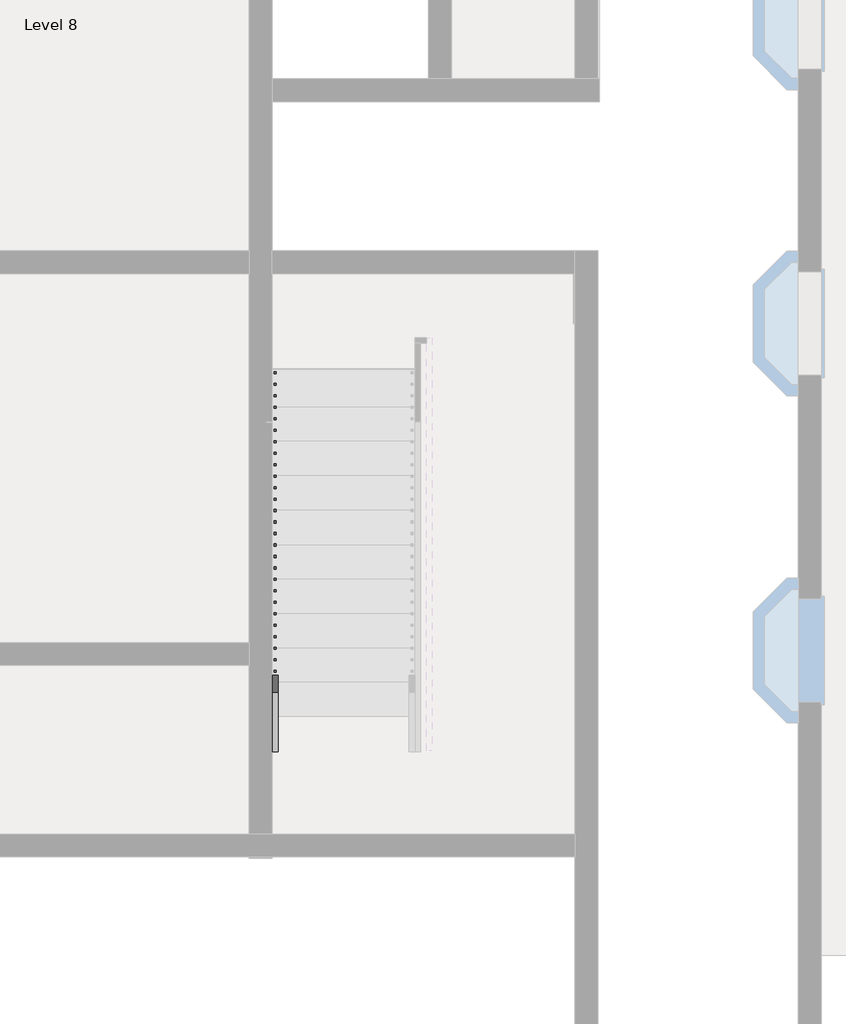
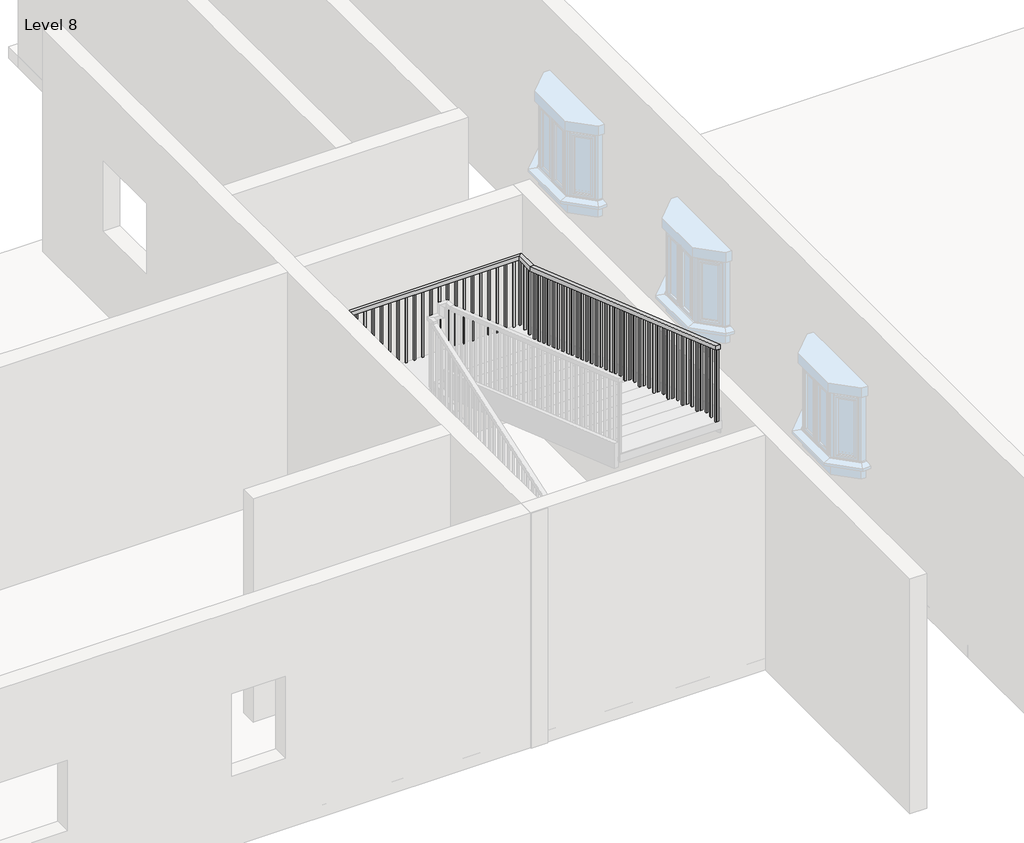
# One storey, part 8 of 14: 1 railing.
"""IFC4 building model written with IfcOpenShell, lengths in millimetres."""

from ifc_helpers import new_model, si_unit, frame, origin, place, context, project, spatial, polyline, outline, extrude, faceted_brep, element, save

model = new_model("IFC4")

# Units and contexts
model_context = context("Model", 3, world=origin())
ifc_project = project(units=[si_unit("LENGTHUNIT", "METRE", prefix="MILLI")], contexts=[model_context])

# Site, building, storey
site = spatial("IfcSite", under=ifc_project)
building = spatial("IfcBuilding", under=site)
storey = spatial("IfcBuildingStorey", under=building, Name="Level 8", Elevation=21336.0)

# Railing
placement = place(None, origin())
element("IfcRailing", 1, ObjectType="Handrail - Rectangular", at=placement, inside=storey, context=model_context, shape_type="SolidModel", body=[
    faceted_brep([(-3857.687215, -9955.5916506, 22355.9076923), (-3857.687215, -9955.5916506, 22302.1602476), (-3806.887215, -9955.5916506, 22302.1602476), (-3806.887215, -9955.5916506, 22355.9076923), (-3857.687215, -6291.6416506, 23622.0), (-3857.687215, -6283.1120276, 23571.2), (-3806.887215, -6283.1120276, 23571.2), (-3806.887215, -6291.6416506, 23622.0), (-3857.687215, -5713.7916506, 23622.0), (-3857.687215, -5713.7916506, 23571.2), (-3806.887215, -5764.5916506, 23571.2), (-3806.887215, -5764.5916506, 23622.0), (-1190.687215, -5713.7916506, 23622.0), (-1190.687215, -5713.7916506, 23571.2), (-1241.487215, -5764.5916506, 23571.2), (-1241.487215, -5764.5916506, 23622.0), (-1190.687215, -5986.8416506, 23622.0), (-1190.687215, -5995.3852679, 23571.2), (-1241.487215, -5995.3852679, 23571.2), (-1241.487215, -5986.8416506, 23622.0), (-1190.687215, -9949.2416506, 24993.6), (-1241.487215, -9949.2416506, 24993.6), (-1241.487215, -9949.2416506, 24939.842594), (-1190.687215, -9949.2416506, 24939.842594)], [[[0, 1, 2, 3]], [[1, 0, 4, 5]], [[2, 1, 5, 6]], [[3, 2, 6, 7]], [[0, 3, 7, 4]], [[5, 4, 8, 9]], [[6, 5, 9, 10]], [[7, 6, 10, 11]], [[4, 7, 11, 8]], [[9, 8, 12, 13]], [[10, 9, 13, 14]], [[11, 10, 14, 15]], [[8, 11, 15, 12]], [[13, 12, 16, 17]], [[14, 13, 17, 18]], [[15, 14, 18, 19]], [[12, 15, 19, 16]], [[20, 21, 22, 23]], [[17, 16, 20, 23]], [[18, 17, 23, 22]], [[19, 18, 22, 21]], [[16, 19, 21, 20]]]),
    extrude(outline(polyline([(-9895.2666506, 24921.1589402), (-9895.2666506, 23973.6923077), (-9914.3166506, 23973.6923077), (-9914.3166506, 24927.7531709), (-9895.2666506, 24921.1589402)])), frame((-1225.612215, 0.0, 0.0), z_axis=(1.0, 0.0, 0.0), x_axis=(0.0, 1.0, 0.0)), (0.0, 0.0, 1.0), 19.05),
    extrude(outline(polyline([(-9793.6666506, 24885.9897094), (-9793.6666506, 23973.6923077), (-9812.7166506, 23973.6923077), (-9812.7166506, 24892.5839402), (-9793.6666506, 24885.9897094)])), frame((-1225.612215, 0.0, 0.0), z_axis=(1.0, 0.0, 0.0), x_axis=(0.0, 1.0, 0.0)), (0.0, 0.0, 1.0), 19.05),
    extrude(outline(polyline([(-9692.0666506, 24850.8204786), (-9692.0666506, 23973.6923077), (-9711.1166506, 23973.6923077), (-9711.1166506, 24857.4147094), (-9692.0666506, 24850.8204786)])), frame((-1225.612215, 0.0, 0.0), z_axis=(1.0, 0.0, 0.0), x_axis=(0.0, 1.0, 0.0)), (0.0, 0.0, 1.0), 19.05),
    extrude(outline(polyline([(-9590.4666506, 24815.6512479), (-9590.4666506, 23868.1846154), (-9609.5166506, 23868.1846154), (-9609.5166506, 24822.2454786), (-9590.4666506, 24815.6512479)])), frame((-1225.612215, 0.0, 0.0), z_axis=(1.0, 0.0, 0.0), x_axis=(0.0, 1.0, 0.0)), (0.0, 0.0, 1.0), 19.05),
    extrude(outline(polyline([(-9488.8666506, 24780.4820171), (-9488.8666506, 23868.1846154), (-9507.9166506, 23868.1846154), (-9507.9166506, 24787.0762479), (-9488.8666506, 24780.4820171)])), frame((-1225.612215, 0.0, 0.0), z_axis=(1.0, 0.0, 0.0), x_axis=(0.0, 1.0, 0.0)), (0.0, 0.0, 1.0), 19.05),
    extrude(outline(polyline([(-9387.2666506, 24745.3127863), (-9387.2666506, 23868.1846154), (-9406.3166506, 23868.1846154), (-9406.3166506, 24751.9070171), (-9387.2666506, 24745.3127863)])), frame((-1225.612215, 0.0, 0.0), z_axis=(1.0, 0.0, 0.0), x_axis=(0.0, 1.0, 0.0)), (0.0, 0.0, 1.0), 19.05),
    extrude(outline(polyline([(-9285.6666506, 24710.1435556), (-9285.6666506, 23762.6769231), (-9304.7166506, 23762.6769231), (-9304.7166506, 24716.7377863), (-9285.6666506, 24710.1435556)])), frame((-1225.612215, 0.0, 0.0), z_axis=(1.0, 0.0, 0.0), x_axis=(0.0, 1.0, 0.0)), (0.0, 0.0, 1.0), 19.05),
    extrude(outline(polyline([(-9184.0666506, 24674.9743248), (-9184.0666506, 23762.6769231), (-9203.1166506, 23762.6769231), (-9203.1166506, 24681.5685556), (-9184.0666506, 24674.9743248)])), frame((-1225.612215, 0.0, 0.0), z_axis=(1.0, 0.0, 0.0), x_axis=(0.0, 1.0, 0.0)), (0.0, 0.0, 1.0), 19.05),
    extrude(outline(polyline([(-9082.4666506, 24639.805094), (-9082.4666506, 23762.6769231), (-9101.5166506, 23762.6769231), (-9101.5166506, 24646.3993248), (-9082.4666506, 24639.805094)])), frame((-1225.612215, 0.0, 0.0), z_axis=(1.0, 0.0, 0.0), x_axis=(0.0, 1.0, 0.0)), (0.0, 0.0, 1.0), 19.05),
    extrude(outline(polyline([(-8980.8666506, 24604.6358632), (-8980.8666506, 23657.1692308), (-8999.9166506, 23657.1692308), (-8999.9166506, 24611.230094), (-8980.8666506, 24604.6358632)])), frame((-1225.612215, 0.0, 0.0), z_axis=(1.0, 0.0, 0.0), x_axis=(0.0, 1.0, 0.0)), (0.0, 0.0, 1.0), 19.05),
    extrude(outline(polyline([(-8879.2666506, 24569.4666325), (-8879.2666506, 23657.1692308), (-8898.3166506, 23657.1692308), (-8898.3166506, 24576.0608632), (-8879.2666506, 24569.4666325)])), frame((-1225.612215, 0.0, 0.0), z_axis=(1.0, 0.0, 0.0), x_axis=(0.0, 1.0, 0.0)), (0.0, 0.0, 1.0), 19.05),
    extrude(outline(polyline([(-8777.6666506, 24534.2974017), (-8777.6666506, 23657.1692308), (-8796.7166506, 23657.1692308), (-8796.7166506, 24540.8916325), (-8777.6666506, 24534.2974017)])), frame((-1225.612215, 0.0, 0.0), z_axis=(1.0, 0.0, 0.0), x_axis=(0.0, 1.0, 0.0)), (0.0, 0.0, 1.0), 19.05),
    extrude(outline(polyline([(-8676.0666506, 24499.1281709), (-8676.0666506, 23551.6615385), (-8695.1166506, 23551.6615385), (-8695.1166506, 24505.7224017), (-8676.0666506, 24499.1281709)])), frame((-1225.612215, 0.0, 0.0), z_axis=(1.0, 0.0, 0.0), x_axis=(0.0, 1.0, 0.0)), (0.0, 0.0, 1.0), 19.05),
    extrude(outline(polyline([(-8574.4666506, 24463.9589402), (-8574.4666506, 23551.6615385), (-8593.5166506, 23551.6615385), (-8593.5166506, 24470.5531709), (-8574.4666506, 24463.9589402)])), frame((-1225.612215, 0.0, 0.0), z_axis=(1.0, 0.0, 0.0), x_axis=(0.0, 1.0, 0.0)), (0.0, 0.0, 1.0), 19.05),
    extrude(outline(polyline([(-8472.8666506, 24428.7897094), (-8472.8666506, 23551.6615385), (-8491.9166506, 23551.6615385), (-8491.9166506, 24435.3839402), (-8472.8666506, 24428.7897094)])), frame((-1225.612215, 0.0, 0.0), z_axis=(1.0, 0.0, 0.0), x_axis=(0.0, 1.0, 0.0)), (0.0, 0.0, 1.0), 19.05),
    extrude(outline(polyline([(-8371.2666506, 24393.6204786), (-8371.2666506, 23446.1538462), (-8390.3166506, 23446.1538462), (-8390.3166506, 24400.2147094), (-8371.2666506, 24393.6204786)])), frame((-1225.612215, 0.0, 0.0), z_axis=(1.0, 0.0, 0.0), x_axis=(0.0, 1.0, 0.0)), (0.0, 0.0, 1.0), 19.05),
    extrude(outline(polyline([(-8269.6666506, 24358.4512479), (-8269.6666506, 23446.1538462), (-8288.7166506, 23446.1538462), (-8288.7166506, 24365.0454786), (-8269.6666506, 24358.4512479)])), frame((-1225.612215, 0.0, 0.0), z_axis=(1.0, 0.0, 0.0), x_axis=(0.0, 1.0, 0.0)), (0.0, 0.0, 1.0), 19.05),
    extrude(outline(polyline([(-8168.0666506, 24323.2820171), (-8168.0666506, 23446.1538462), (-8187.1166506, 23446.1538462), (-8187.1166506, 24329.8762479), (-8168.0666506, 24323.2820171)])), frame((-1225.612215, 0.0, 0.0), z_axis=(1.0, 0.0, 0.0), x_axis=(0.0, 1.0, 0.0)), (0.0, 0.0, 1.0), 19.05),
    extrude(outline(polyline([(-8066.4666506, 24288.1127863), (-8066.4666506, 23340.6461538), (-8085.5166506, 23340.6461538), (-8085.5166506, 24294.7070171), (-8066.4666506, 24288.1127863)])), frame((-1225.612215, 0.0, 0.0), z_axis=(1.0, 0.0, 0.0), x_axis=(0.0, 1.0, 0.0)), (0.0, 0.0, 1.0), 19.05),
    extrude(outline(polyline([(-7964.8666506, 24252.9435556), (-7964.8666506, 23340.6461538), (-7983.9166506, 23340.6461538), (-7983.9166506, 24259.5377863), (-7964.8666506, 24252.9435556)])), frame((-1225.612215, 0.0, 0.0), z_axis=(1.0, 0.0, 0.0), x_axis=(0.0, 1.0, 0.0)), (0.0, 0.0, 1.0), 19.05),
    extrude(outline(polyline([(-7863.2666506, 24217.7743248), (-7863.2666506, 23340.6461538), (-7882.3166506, 23340.6461538), (-7882.3166506, 24224.3685556), (-7863.2666506, 24217.7743248)])), frame((-1225.612215, 0.0, 0.0), z_axis=(1.0, 0.0, 0.0), x_axis=(0.0, 1.0, 0.0)), (0.0, 0.0, 1.0), 19.05),
    extrude(outline(polyline([(-7761.6666506, 24182.605094), (-7761.6666506, 23235.1384615), (-7780.7166506, 23235.1384615), (-7780.7166506, 24189.1993248), (-7761.6666506, 24182.605094)])), frame((-1225.612215, 0.0, 0.0), z_axis=(1.0, 0.0, 0.0), x_axis=(0.0, 1.0, 0.0)), (0.0, 0.0, 1.0), 19.05),
    extrude(outline(polyline([(-7660.0666506, 24147.4358632), (-7660.0666506, 23235.1384615), (-7679.1166506, 23235.1384615), (-7679.1166506, 24154.030094), (-7660.0666506, 24147.4358632)])), frame((-1225.612215, 0.0, 0.0), z_axis=(1.0, 0.0, 0.0), x_axis=(0.0, 1.0, 0.0)), (0.0, 0.0, 1.0), 19.05),
    extrude(outline(polyline([(-7558.4666506, 24112.2666325), (-7558.4666506, 23235.1384615), (-7577.5166506, 23235.1384615), (-7577.5166506, 24118.8608632), (-7558.4666506, 24112.2666325)])), frame((-1225.612215, 0.0, 0.0), z_axis=(1.0, 0.0, 0.0), x_axis=(0.0, 1.0, 0.0)), (0.0, 0.0, 1.0), 19.05),
    extrude(outline(polyline([(-7456.8666506, 24077.0974017), (-7456.8666506, 23129.6307692), (-7475.9166506, 23129.6307692), (-7475.9166506, 24083.6916325), (-7456.8666506, 24077.0974017)])), frame((-1225.612215, 0.0, 0.0), z_axis=(1.0, 0.0, 0.0), x_axis=(0.0, 1.0, 0.0)), (0.0, 0.0, 1.0), 19.05),
    extrude(outline(polyline([(-7355.2666506, 24041.9281709), (-7355.2666506, 23129.6307692), (-7374.3166506, 23129.6307692), (-7374.3166506, 24048.5224017), (-7355.2666506, 24041.9281709)])), frame((-1225.612215, 0.0, 0.0), z_axis=(1.0, 0.0, 0.0), x_axis=(0.0, 1.0, 0.0)), (0.0, 0.0, 1.0), 19.05),
    extrude(outline(polyline([(-7253.6666506, 24006.7589402), (-7253.6666506, 23129.6307692), (-7272.7166506, 23129.6307692), (-7272.7166506, 24013.3531709), (-7253.6666506, 24006.7589402)])), frame((-1225.612215, 0.0, 0.0), z_axis=(1.0, 0.0, 0.0), x_axis=(0.0, 1.0, 0.0)), (0.0, 0.0, 1.0), 19.05),
    extrude(outline(polyline([(-7152.0666506, 23971.5897094), (-7152.0666506, 23024.1230769), (-7171.1166506, 23024.1230769), (-7171.1166506, 23978.1839402), (-7152.0666506, 23971.5897094)])), frame((-1225.612215, 0.0, 0.0), z_axis=(1.0, 0.0, 0.0), x_axis=(0.0, 1.0, 0.0)), (0.0, 0.0, 1.0), 19.05),
    extrude(outline(polyline([(-7050.4666506, 23936.4204786), (-7050.4666506, 23024.1230769), (-7069.5166506, 23024.1230769), (-7069.5166506, 23943.0147094), (-7050.4666506, 23936.4204786)])), frame((-1225.612215, 0.0, 0.0), z_axis=(1.0, 0.0, 0.0), x_axis=(0.0, 1.0, 0.0)), (0.0, 0.0, 1.0), 19.05),
    extrude(outline(polyline([(-6948.8666506, 23901.2512479), (-6948.8666506, 23024.1230769), (-6967.9166506, 23024.1230769), (-6967.9166506, 23907.8454786), (-6948.8666506, 23901.2512479)])), frame((-1225.612215, 0.0, 0.0), z_axis=(1.0, 0.0, 0.0), x_axis=(0.0, 1.0, 0.0)), (0.0, 0.0, 1.0), 19.05),
    extrude(outline(polyline([(-6847.2666506, 23866.0820171), (-6847.2666506, 22918.6153846), (-6866.3166506, 22918.6153846), (-6866.3166506, 23872.6762479), (-6847.2666506, 23866.0820171)])), frame((-1225.612215, 0.0, 0.0), z_axis=(1.0, 0.0, 0.0), x_axis=(0.0, 1.0, 0.0)), (0.0, 0.0, 1.0), 19.05),
    extrude(outline(polyline([(-6745.6666506, 23830.9127863), (-6745.6666506, 22918.6153846), (-6764.7166506, 22918.6153846), (-6764.7166506, 23837.5070171), (-6745.6666506, 23830.9127863)])), frame((-1225.612215, 0.0, 0.0), z_axis=(1.0, 0.0, 0.0), x_axis=(0.0, 1.0, 0.0)), (0.0, 0.0, 1.0), 19.05),
    extrude(outline(polyline([(-6644.0666506, 23795.7435556), (-6644.0666506, 22918.6153846), (-6663.1166506, 22918.6153846), (-6663.1166506, 23802.3377863), (-6644.0666506, 23795.7435556)])), frame((-1225.612215, 0.0, 0.0), z_axis=(1.0, 0.0, 0.0), x_axis=(0.0, 1.0, 0.0)), (0.0, 0.0, 1.0), 19.05),
    extrude(outline(polyline([(-6542.4666506, 23760.5743248), (-6542.4666506, 22813.1076923), (-6561.5166506, 22813.1076923), (-6561.5166506, 23767.1685556), (-6542.4666506, 23760.5743248)])), frame((-1225.612215, 0.0, 0.0), z_axis=(1.0, 0.0, 0.0), x_axis=(0.0, 1.0, 0.0)), (0.0, 0.0, 1.0), 19.05),
    extrude(outline(polyline([(-6440.8666506, 23725.405094), (-6440.8666506, 22813.1076923), (-6459.9166506, 22813.1076923), (-6459.9166506, 23731.9993248), (-6440.8666506, 23725.405094)])), frame((-1225.612215, 0.0, 0.0), z_axis=(1.0, 0.0, 0.0), x_axis=(0.0, 1.0, 0.0)), (0.0, 0.0, 1.0), 19.05),
    extrude(outline(polyline([(-6339.2666506, 23690.2358632), (-6339.2666506, 22813.1076923), (-6358.3166506, 22813.1076923), (-6358.3166506, 23696.830094), (-6339.2666506, 23690.2358632)])), frame((-1225.612215, 0.0, 0.0), z_axis=(1.0, 0.0, 0.0), x_axis=(0.0, 1.0, 0.0)), (0.0, 0.0, 1.0), 19.05),
    extrude(outline(polyline([(-6237.6666506, 23655.0666325), (-6237.6666506, 22707.6), (-6256.7166506, 22707.6), (-6256.7166506, 23661.6608632), (-6237.6666506, 23655.0666325)])), frame((-1225.612215, 0.0, 0.0), z_axis=(1.0, 0.0, 0.0), x_axis=(0.0, 1.0, 0.0)), (0.0, 0.0, 1.0), 19.05),
    extrude(outline(polyline([(-6136.0666506, 23619.8974017), (-6136.0666506, 22707.6), (-6155.1166506, 22707.6), (-6155.1166506, 23626.4916325), (-6136.0666506, 23619.8974017)])), frame((-1225.612215, 0.0, 0.0), z_axis=(1.0, 0.0, 0.0), x_axis=(0.0, 1.0, 0.0)), (0.0, 0.0, 1.0), 19.05),
    extrude(outline(polyline([(-6034.4666506, 23584.7281709), (-6034.4666506, 22707.6), (-6053.5166506, 22707.6), (-6053.5166506, 23591.3224017), (-6034.4666506, 23584.7281709)])), frame((-1225.612215, 0.0, 0.0), z_axis=(1.0, 0.0, 0.0), x_axis=(0.0, 1.0, 0.0)), (0.0, 0.0, 1.0), 19.05),
    extrude(outline(polyline([(-1206.562215, -5932.8666506), (-1206.562215, -5951.9166506), (-1225.612215, -5951.9166506), (-1225.612215, -5932.8666506), (-1206.562215, -5932.8666506)])), frame((0.0, 0.0, 22707.6), z_axis=(0.0, 0.0, 1.0), x_axis=(1.0, 0.0, 0.0)), (0.0, 0.0, 1.0), 863.6),
    extrude(outline(polyline([(-1206.562215, -5831.2666506), (-1206.562215, -5850.3166506), (-1225.612215, -5850.3166506), (-1225.612215, -5831.2666506), (-1206.562215, -5831.2666506)])), frame((0.0, 0.0, 22707.6), z_axis=(0.0, 0.0, 1.0), x_axis=(1.0, 0.0, 0.0)), (0.0, 0.0, 1.0), 863.6),
    extrude(outline(polyline([(-1301.812215, -5729.6666506), (-1282.762215, -5729.6666506), (-1282.762215, -5748.7166506), (-1301.812215, -5748.7166506), (-1301.812215, -5729.6666506)])), frame((0.0, 0.0, 22707.6), z_axis=(0.0, 0.0, 1.0), x_axis=(1.0, 0.0, 0.0)), (0.0, 0.0, 1.0), 863.6),
    extrude(outline(polyline([(-1403.412215, -5729.6666506), (-1384.362215, -5729.6666506), (-1384.362215, -5748.7166506), (-1403.412215, -5748.7166506), (-1403.412215, -5729.6666506)])), frame((0.0, 0.0, 22707.6), z_axis=(0.0, 0.0, 1.0), x_axis=(1.0, 0.0, 0.0)), (0.0, 0.0, 1.0), 863.6),
    extrude(outline(polyline([(-1505.012215, -5729.6666506), (-1485.962215, -5729.6666506), (-1485.962215, -5748.7166506), (-1505.012215, -5748.7166506), (-1505.012215, -5729.6666506)])), frame((0.0, 0.0, 22707.6), z_axis=(0.0, 0.0, 1.0), x_axis=(1.0, 0.0, 0.0)), (0.0, 0.0, 1.0), 863.6),
    extrude(outline(polyline([(-1606.612215, -5729.6666506), (-1587.562215, -5729.6666506), (-1587.562215, -5748.7166506), (-1606.612215, -5748.7166506), (-1606.612215, -5729.6666506)])), frame((0.0, 0.0, 22707.6), z_axis=(0.0, 0.0, 1.0), x_axis=(1.0, 0.0, 0.0)), (0.0, 0.0, 1.0), 863.6),
    extrude(outline(polyline([(-1708.212215, -5729.6666506), (-1689.162215, -5729.6666506), (-1689.162215, -5748.7166506), (-1708.212215, -5748.7166506), (-1708.212215, -5729.6666506)])), frame((0.0, 0.0, 22707.6), z_axis=(0.0, 0.0, 1.0), x_axis=(1.0, 0.0, 0.0)), (0.0, 0.0, 1.0), 863.6),
    extrude(outline(polyline([(-1809.812215, -5729.6666506), (-1790.762215, -5729.6666506), (-1790.762215, -5748.7166506), (-1809.812215, -5748.7166506), (-1809.812215, -5729.6666506)])), frame((0.0, 0.0, 22707.6), z_axis=(0.0, 0.0, 1.0), x_axis=(1.0, 0.0, 0.0)), (0.0, 0.0, 1.0), 863.6),
    extrude(outline(polyline([(-1911.412215, -5729.6666506), (-1892.362215, -5729.6666506), (-1892.362215, -5748.7166506), (-1911.412215, -5748.7166506), (-1911.412215, -5729.6666506)])), frame((0.0, 0.0, 22707.6), z_axis=(0.0, 0.0, 1.0), x_axis=(1.0, 0.0, 0.0)), (0.0, 0.0, 1.0), 863.6),
    extrude(outline(polyline([(-2013.012215, -5729.6666506), (-1993.962215, -5729.6666506), (-1993.962215, -5748.7166506), (-2013.012215, -5748.7166506), (-2013.012215, -5729.6666506)])), frame((0.0, 0.0, 22707.6), z_axis=(0.0, 0.0, 1.0), x_axis=(1.0, 0.0, 0.0)), (0.0, 0.0, 1.0), 863.6),
    extrude(outline(polyline([(-2114.612215, -5729.6666506), (-2095.562215, -5729.6666506), (-2095.562215, -5748.7166506), (-2114.612215, -5748.7166506), (-2114.612215, -5729.6666506)])), frame((0.0, 0.0, 22707.6), z_axis=(0.0, 0.0, 1.0), x_axis=(1.0, 0.0, 0.0)), (0.0, 0.0, 1.0), 863.6),
    extrude(outline(polyline([(-2216.212215, -5729.6666506), (-2197.162215, -5729.6666506), (-2197.162215, -5748.7166506), (-2216.212215, -5748.7166506), (-2216.212215, -5729.6666506)])), frame((0.0, 0.0, 22707.6), z_axis=(0.0, 0.0, 1.0), x_axis=(1.0, 0.0, 0.0)), (0.0, 0.0, 1.0), 863.6),
    extrude(outline(polyline([(-2317.812215, -5729.6666506), (-2298.762215, -5729.6666506), (-2298.762215, -5748.7166506), (-2317.812215, -5748.7166506), (-2317.812215, -5729.6666506)])), frame((0.0, 0.0, 22707.6), z_axis=(0.0, 0.0, 1.0), x_axis=(1.0, 0.0, 0.0)), (0.0, 0.0, 1.0), 863.6),
    extrude(outline(polyline([(-2419.412215, -5729.6666506), (-2400.362215, -5729.6666506), (-2400.362215, -5748.7166506), (-2419.412215, -5748.7166506), (-2419.412215, -5729.6666506)])), frame((0.0, 0.0, 22707.6), z_axis=(0.0, 0.0, 1.0), x_axis=(1.0, 0.0, 0.0)), (0.0, 0.0, 1.0), 863.6),
    extrude(outline(polyline([(-2521.012215, -5729.6666506), (-2501.962215, -5729.6666506), (-2501.962215, -5748.7166506), (-2521.012215, -5748.7166506), (-2521.012215, -5729.6666506)])), frame((0.0, 0.0, 22707.6), z_axis=(0.0, 0.0, 1.0), x_axis=(1.0, 0.0, 0.0)), (0.0, 0.0, 1.0), 863.6),
    extrude(outline(polyline([(-2622.612215, -5729.6666506), (-2603.562215, -5729.6666506), (-2603.562215, -5748.7166506), (-2622.612215, -5748.7166506), (-2622.612215, -5729.6666506)])), frame((0.0, 0.0, 22707.6), z_axis=(0.0, 0.0, 1.0), x_axis=(1.0, 0.0, 0.0)), (0.0, 0.0, 1.0), 863.6),
    extrude(outline(polyline([(-2724.212215, -5729.6666506), (-2705.162215, -5729.6666506), (-2705.162215, -5748.7166506), (-2724.212215, -5748.7166506), (-2724.212215, -5729.6666506)])), frame((0.0, 0.0, 22707.6), z_axis=(0.0, 0.0, 1.0), x_axis=(1.0, 0.0, 0.0)), (0.0, 0.0, 1.0), 863.6),
    extrude(outline(polyline([(-2825.812215, -5729.6666506), (-2806.762215, -5729.6666506), (-2806.762215, -5748.7166506), (-2825.812215, -5748.7166506), (-2825.812215, -5729.6666506)])), frame((0.0, 0.0, 22707.6), z_axis=(0.0, 0.0, 1.0), x_axis=(1.0, 0.0, 0.0)), (0.0, 0.0, 1.0), 863.6),
    extrude(outline(polyline([(-2927.412215, -5729.6666506), (-2908.362215, -5729.6666506), (-2908.362215, -5748.7166506), (-2927.412215, -5748.7166506), (-2927.412215, -5729.6666506)])), frame((0.0, 0.0, 22707.6), z_axis=(0.0, 0.0, 1.0), x_axis=(1.0, 0.0, 0.0)), (0.0, 0.0, 1.0), 863.6),
    extrude(outline(polyline([(-3029.012215, -5729.6666506), (-3009.962215, -5729.6666506), (-3009.962215, -5748.7166506), (-3029.012215, -5748.7166506), (-3029.012215, -5729.6666506)])), frame((0.0, 0.0, 22707.6), z_axis=(0.0, 0.0, 1.0), x_axis=(1.0, 0.0, 0.0)), (0.0, 0.0, 1.0), 863.6),
    extrude(outline(polyline([(-3130.612215, -5729.6666506), (-3111.562215, -5729.6666506), (-3111.562215, -5748.7166506), (-3130.612215, -5748.7166506), (-3130.612215, -5729.6666506)])), frame((0.0, 0.0, 22707.6), z_axis=(0.0, 0.0, 1.0), x_axis=(1.0, 0.0, 0.0)), (0.0, 0.0, 1.0), 863.6),
    extrude(outline(polyline([(-3232.212215, -5729.6666506), (-3213.162215, -5729.6666506), (-3213.162215, -5748.7166506), (-3232.212215, -5748.7166506), (-3232.212215, -5729.6666506)])), frame((0.0, 0.0, 22707.6), z_axis=(0.0, 0.0, 1.0), x_axis=(1.0, 0.0, 0.0)), (0.0, 0.0, 1.0), 863.6),
    extrude(outline(polyline([(-3333.812215, -5729.6666506), (-3314.762215, -5729.6666506), (-3314.762215, -5748.7166506), (-3333.812215, -5748.7166506), (-3333.812215, -5729.6666506)])), frame((0.0, 0.0, 22707.6), z_axis=(0.0, 0.0, 1.0), x_axis=(1.0, 0.0, 0.0)), (0.0, 0.0, 1.0), 863.6),
    extrude(outline(polyline([(-3435.412215, -5729.6666506), (-3416.362215, -5729.6666506), (-3416.362215, -5748.7166506), (-3435.412215, -5748.7166506), (-3435.412215, -5729.6666506)])), frame((0.0, 0.0, 22707.6), z_axis=(0.0, 0.0, 1.0), x_axis=(1.0, 0.0, 0.0)), (0.0, 0.0, 1.0), 863.6),
    extrude(outline(polyline([(-3537.012215, -5729.6666506), (-3517.962215, -5729.6666506), (-3517.962215, -5748.7166506), (-3537.012215, -5748.7166506), (-3537.012215, -5729.6666506)])), frame((0.0, 0.0, 22707.6), z_axis=(0.0, 0.0, 1.0), x_axis=(1.0, 0.0, 0.0)), (0.0, 0.0, 1.0), 863.6),
    extrude(outline(polyline([(-3638.612215, -5729.6666506), (-3619.562215, -5729.6666506), (-3619.562215, -5748.7166506), (-3638.612215, -5748.7166506), (-3638.612215, -5729.6666506)])), frame((0.0, 0.0, 22707.6), z_axis=(0.0, 0.0, 1.0), x_axis=(1.0, 0.0, 0.0)), (0.0, 0.0, 1.0), 863.6),
    extrude(outline(polyline([(-3740.212215, -5729.6666506), (-3721.162215, -5729.6666506), (-3721.162215, -5748.7166506), (-3740.212215, -5748.7166506), (-3740.212215, -5729.6666506)])), frame((0.0, 0.0, 22707.6), z_axis=(0.0, 0.0, 1.0), x_axis=(1.0, 0.0, 0.0)), (0.0, 0.0, 1.0), 863.6),
    extrude(outline(polyline([(-3841.812215, -5799.5166506), (-3841.812215, -5780.4666506), (-3822.762215, -5780.4666506), (-3822.762215, -5799.5166506), (-3841.812215, -5799.5166506)])), frame((0.0, 0.0, 22707.6), z_axis=(0.0, 0.0, 1.0), x_axis=(1.0, 0.0, 0.0)), (0.0, 0.0, 1.0), 863.6),
    extrude(outline(polyline([(-3841.812215, -5901.1166506), (-3841.812215, -5882.0666506), (-3822.762215, -5882.0666506), (-3822.762215, -5901.1166506), (-3841.812215, -5901.1166506)])), frame((0.0, 0.0, 22707.6), z_axis=(0.0, 0.0, 1.0), x_axis=(1.0, 0.0, 0.0)), (0.0, 0.0, 1.0), 863.6),
    extrude(outline(polyline([(-3841.812215, -6002.7166506), (-3841.812215, -5983.6666506), (-3822.762215, -5983.6666506), (-3822.762215, -6002.7166506), (-3841.812215, -6002.7166506)])), frame((0.0, 0.0, 22707.6), z_axis=(0.0, 0.0, 1.0), x_axis=(1.0, 0.0, 0.0)), (0.0, 0.0, 1.0), 863.6),
    extrude(outline(polyline([(-3841.812215, -6104.3166506), (-3841.812215, -6085.2666506), (-3822.762215, -6085.2666506), (-3822.762215, -6104.3166506), (-3841.812215, -6104.3166506)])), frame((0.0, 0.0, 22707.6), z_axis=(0.0, 0.0, 1.0), x_axis=(1.0, 0.0, 0.0)), (0.0, 0.0, 1.0), 863.6),
    extrude(outline(polyline([(-3841.812215, -6205.9166506), (-3841.812215, -6186.8666506), (-3822.762215, -6186.8666506), (-3822.762215, -6205.9166506), (-3841.812215, -6205.9166506)])), frame((0.0, 0.0, 22707.6), z_axis=(0.0, 0.0, 1.0), x_axis=(1.0, 0.0, 0.0)), (0.0, 0.0, 1.0), 863.6),
    extrude(outline(polyline([(-6288.4666506, 23569.349689), (-6288.4666506, 22602.0923077), (-6307.5166506, 22602.0923077), (-6307.5166506, 23562.7668867), (-6288.4666506, 23569.349689)])), frame((-3841.812215, 0.0, 0.0), z_axis=(1.0, 0.0, 0.0), x_axis=(0.0, 1.0, 0.0)), (0.0, 0.0, 1.0), 19.05),
    extrude(outline(polyline([(-6390.0666506, 23534.2414101), (-6390.0666506, 22602.0923077), (-6409.1166506, 22602.0923077), (-6409.1166506, 23527.6586078), (-6390.0666506, 23534.2414101)])), frame((-3841.812215, 0.0, 0.0), z_axis=(1.0, 0.0, 0.0), x_axis=(0.0, 1.0, 0.0)), (0.0, 0.0, 1.0), 19.05),
    extrude(outline(polyline([(-6491.6666506, 23499.1331312), (-6491.6666506, 22602.0923077), (-6510.7166506, 22602.0923077), (-6510.7166506, 23492.5503289), (-6491.6666506, 23499.1331312)])), frame((-3841.812215, 0.0, 0.0), z_axis=(1.0, 0.0, 0.0), x_axis=(0.0, 1.0, 0.0)), (0.0, 0.0, 1.0), 19.05),
    extrude(outline(polyline([(-6593.2666506, 23464.0248523), (-6593.2666506, 22496.5846154), (-6612.3166506, 22496.5846154), (-6612.3166506, 23457.44205), (-6593.2666506, 23464.0248523)])), frame((-3841.812215, 0.0, 0.0), z_axis=(1.0, 0.0, 0.0), x_axis=(0.0, 1.0, 0.0)), (0.0, 0.0, 1.0), 19.05),
    extrude(outline(polyline([(-6694.8666506, 23428.9165734), (-6694.8666506, 22496.5846154), (-6713.9166506, 22496.5846154), (-6713.9166506, 23422.3337711), (-6694.8666506, 23428.9165734)])), frame((-3841.812215, 0.0, 0.0), z_axis=(1.0, 0.0, 0.0), x_axis=(0.0, 1.0, 0.0)), (0.0, 0.0, 1.0), 19.05),
    extrude(outline(polyline([(-6796.4666506, 23393.8082945), (-6796.4666506, 22496.5846154), (-6815.5166506, 22496.5846154), (-6815.5166506, 23387.2254922), (-6796.4666506, 23393.8082945)])), frame((-3841.812215, 0.0, 0.0), z_axis=(1.0, 0.0, 0.0), x_axis=(0.0, 1.0, 0.0)), (0.0, 0.0, 1.0), 19.05),
    extrude(outline(polyline([(-6898.0666506, 23358.7000156), (-6898.0666506, 22391.0769231), (-6917.1166506, 22391.0769231), (-6917.1166506, 23352.1172133), (-6898.0666506, 23358.7000156)])), frame((-3841.812215, 0.0, 0.0), z_axis=(1.0, 0.0, 0.0), x_axis=(0.0, 1.0, 0.0)), (0.0, 0.0, 1.0), 19.05),
    extrude(outline(polyline([(-6999.6666506, 23323.5917367), (-6999.6666506, 22391.0769231), (-7018.7166506, 22391.0769231), (-7018.7166506, 23317.0089344), (-6999.6666506, 23323.5917367)])), frame((-3841.812215, 0.0, 0.0), z_axis=(1.0, 0.0, 0.0), x_axis=(0.0, 1.0, 0.0)), (0.0, 0.0, 1.0), 19.05),
    extrude(outline(polyline([(-7101.2666506, 23288.4834578), (-7101.2666506, 22391.0769231), (-7120.3166506, 22391.0769231), (-7120.3166506, 23281.9006556), (-7101.2666506, 23288.4834578)])), frame((-3841.812215, 0.0, 0.0), z_axis=(1.0, 0.0, 0.0), x_axis=(0.0, 1.0, 0.0)), (0.0, 0.0, 1.0), 19.05),
    extrude(outline(polyline([(-7202.8666506, 23253.375179), (-7202.8666506, 22285.5692308), (-7221.9166506, 22285.5692308), (-7221.9166506, 23246.7923767), (-7202.8666506, 23253.375179)])), frame((-3841.812215, 0.0, 0.0), z_axis=(1.0, 0.0, 0.0), x_axis=(0.0, 1.0, 0.0)), (0.0, 0.0, 1.0), 19.05),
    extrude(outline(polyline([(-7304.4666506, 23218.2669001), (-7304.4666506, 22285.5692308), (-7323.5166506, 22285.5692308), (-7323.5166506, 23211.6840978), (-7304.4666506, 23218.2669001)])), frame((-3841.812215, 0.0, 0.0), z_axis=(1.0, 0.0, 0.0), x_axis=(0.0, 1.0, 0.0)), (0.0, 0.0, 1.0), 19.05),
    extrude(outline(polyline([(-7406.0666506, 23183.1586212), (-7406.0666506, 22285.5692308), (-7425.1166506, 22285.5692308), (-7425.1166506, 23176.5758189), (-7406.0666506, 23183.1586212)])), frame((-3841.812215, 0.0, 0.0), z_axis=(1.0, 0.0, 0.0), x_axis=(0.0, 1.0, 0.0)), (0.0, 0.0, 1.0), 19.05),
    extrude(outline(polyline([(-7507.6666506, 23148.0503423), (-7507.6666506, 22180.0615385), (-7526.7166506, 22180.0615385), (-7526.7166506, 23141.46754), (-7507.6666506, 23148.0503423)])), frame((-3841.812215, 0.0, 0.0), z_axis=(1.0, 0.0, 0.0), x_axis=(0.0, 1.0, 0.0)), (0.0, 0.0, 1.0), 19.05),
    extrude(outline(polyline([(-7609.2666506, 23112.9420634), (-7609.2666506, 22180.0615385), (-7628.3166506, 22180.0615385), (-7628.3166506, 23106.3592611), (-7609.2666506, 23112.9420634)])), frame((-3841.812215, 0.0, 0.0), z_axis=(1.0, 0.0, 0.0), x_axis=(0.0, 1.0, 0.0)), (0.0, 0.0, 1.0), 19.05),
    extrude(outline(polyline([(-7710.8666506, 23077.8337845), (-7710.8666506, 22180.0615385), (-7729.9166506, 22180.0615385), (-7729.9166506, 23071.2509822), (-7710.8666506, 23077.8337845)])), frame((-3841.812215, 0.0, 0.0), z_axis=(1.0, 0.0, 0.0), x_axis=(0.0, 1.0, 0.0)), (0.0, 0.0, 1.0), 19.05),
    extrude(outline(polyline([(-7812.4666506, 23042.7255056), (-7812.4666506, 22074.5538462), (-7831.5166506, 22074.5538462), (-7831.5166506, 23036.1427033), (-7812.4666506, 23042.7255056)])), frame((-3841.812215, 0.0, 0.0), z_axis=(1.0, 0.0, 0.0), x_axis=(0.0, 1.0, 0.0)), (0.0, 0.0, 1.0), 19.05),
    extrude(outline(polyline([(-7914.0666506, 23007.6172267), (-7914.0666506, 22074.5538462), (-7933.1166506, 22074.5538462), (-7933.1166506, 23001.0344244), (-7914.0666506, 23007.6172267)])), frame((-3841.812215, 0.0, 0.0), z_axis=(1.0, 0.0, 0.0), x_axis=(0.0, 1.0, 0.0)), (0.0, 0.0, 1.0), 19.05),
    extrude(outline(polyline([(-8015.6666506, 22972.5089478), (-8015.6666506, 22074.5538462), (-8034.7166506, 22074.5538462), (-8034.7166506, 22965.9261455), (-8015.6666506, 22972.5089478)])), frame((-3841.812215, 0.0, 0.0), z_axis=(1.0, 0.0, 0.0), x_axis=(0.0, 1.0, 0.0)), (0.0, 0.0, 1.0), 19.05),
    extrude(outline(polyline([(-8117.2666506, 22937.4006689), (-8117.2666506, 21969.0461538), (-8136.3166506, 21969.0461538), (-8136.3166506, 22930.8178666), (-8117.2666506, 22937.4006689)])), frame((-3841.812215, 0.0, 0.0), z_axis=(1.0, 0.0, 0.0), x_axis=(0.0, 1.0, 0.0)), (0.0, 0.0, 1.0), 19.05),
    extrude(outline(polyline([(-8218.8666506, 22902.29239), (-8218.8666506, 21969.0461538), (-8237.9166506, 21969.0461538), (-8237.9166506, 22895.7095877), (-8218.8666506, 22902.29239)])), frame((-3841.812215, 0.0, 0.0), z_axis=(1.0, 0.0, 0.0), x_axis=(0.0, 1.0, 0.0)), (0.0, 0.0, 1.0), 19.05),
    extrude(outline(polyline([(-8320.4666506, 22867.1841111), (-8320.4666506, 21969.0461538), (-8339.5166506, 21969.0461538), (-8339.5166506, 22860.6013088), (-8320.4666506, 22867.1841111)])), frame((-3841.812215, 0.0, 0.0), z_axis=(1.0, 0.0, 0.0), x_axis=(0.0, 1.0, 0.0)), (0.0, 0.0, 1.0), 19.05),
    extrude(outline(polyline([(-8422.0666506, 22832.0758322), (-8422.0666506, 21863.5384615), (-8441.1166506, 21863.5384615), (-8441.1166506, 22825.4930299), (-8422.0666506, 22832.0758322)])), frame((-3841.812215, 0.0, 0.0), z_axis=(1.0, 0.0, 0.0), x_axis=(0.0, 1.0, 0.0)), (0.0, 0.0, 1.0), 19.05),
    extrude(outline(polyline([(-8523.6666506, 22796.9675533), (-8523.6666506, 21863.5384615), (-8542.7166506, 21863.5384615), (-8542.7166506, 22790.384751), (-8523.6666506, 22796.9675533)])), frame((-3841.812215, 0.0, 0.0), z_axis=(1.0, 0.0, 0.0), x_axis=(0.0, 1.0, 0.0)), (0.0, 0.0, 1.0), 19.05),
    extrude(outline(polyline([(-8625.2666506, 22761.8592744), (-8625.2666506, 21863.5384615), (-8644.3166506, 21863.5384615), (-8644.3166506, 22755.2764721), (-8625.2666506, 22761.8592744)])), frame((-3841.812215, 0.0, 0.0), z_axis=(1.0, 0.0, 0.0), x_axis=(0.0, 1.0, 0.0)), (0.0, 0.0, 1.0), 19.05),
    extrude(outline(polyline([(-8726.8666506, 22726.7509955), (-8726.8666506, 21758.0307692), (-8745.9166506, 21758.0307692), (-8745.9166506, 22720.1681932), (-8726.8666506, 22726.7509955)])), frame((-3841.812215, 0.0, 0.0), z_axis=(1.0, 0.0, 0.0), x_axis=(0.0, 1.0, 0.0)), (0.0, 0.0, 1.0), 19.05),
    extrude(outline(polyline([(-8828.4666506, 22691.6427166), (-8828.4666506, 21758.0307692), (-8847.5166506, 21758.0307692), (-8847.5166506, 22685.0599143), (-8828.4666506, 22691.6427166)])), frame((-3841.812215, 0.0, 0.0), z_axis=(1.0, 0.0, 0.0), x_axis=(0.0, 1.0, 0.0)), (0.0, 0.0, 1.0), 19.05),
    extrude(outline(polyline([(-8930.0666506, 22656.5344377), (-8930.0666506, 21758.0307692), (-8949.1166506, 21758.0307692), (-8949.1166506, 22649.9516354), (-8930.0666506, 22656.5344377)])), frame((-3841.812215, 0.0, 0.0), z_axis=(1.0, 0.0, 0.0), x_axis=(0.0, 1.0, 0.0)), (0.0, 0.0, 1.0), 19.05),
    extrude(outline(polyline([(-9031.6666506, 22621.4261588), (-9031.6666506, 21652.5230769), (-9050.7166506, 21652.5230769), (-9050.7166506, 22614.8433565), (-9031.6666506, 22621.4261588)])), frame((-3841.812215, 0.0, 0.0), z_axis=(1.0, 0.0, 0.0), x_axis=(0.0, 1.0, 0.0)), (0.0, 0.0, 1.0), 19.05),
    extrude(outline(polyline([(-9133.2666506, 22586.3178799), (-9133.2666506, 21652.5230769), (-9152.3166506, 21652.5230769), (-9152.3166506, 22579.7350776), (-9133.2666506, 22586.3178799)])), frame((-3841.812215, 0.0, 0.0), z_axis=(1.0, 0.0, 0.0), x_axis=(0.0, 1.0, 0.0)), (0.0, 0.0, 1.0), 19.05),
    extrude(outline(polyline([(-9234.8666506, 22551.209601), (-9234.8666506, 21652.5230769), (-9253.9166506, 21652.5230769), (-9253.9166506, 22544.6267987), (-9234.8666506, 22551.209601)])), frame((-3841.812215, 0.0, 0.0), z_axis=(1.0, 0.0, 0.0), x_axis=(0.0, 1.0, 0.0)), (0.0, 0.0, 1.0), 19.05),
    extrude(outline(polyline([(-9336.4666506, 22516.1013221), (-9336.4666506, 21547.0153846), (-9355.5166506, 21547.0153846), (-9355.5166506, 22509.5185198), (-9336.4666506, 22516.1013221)])), frame((-3841.812215, 0.0, 0.0), z_axis=(1.0, 0.0, 0.0), x_axis=(0.0, 1.0, 0.0)), (0.0, 0.0, 1.0), 19.05),
    extrude(outline(polyline([(-9438.0666506, 22480.9930432), (-9438.0666506, 21547.0153846), (-9457.1166506, 21547.0153846), (-9457.1166506, 22474.4102409), (-9438.0666506, 22480.9930432)])), frame((-3841.812215, 0.0, 0.0), z_axis=(1.0, 0.0, 0.0), x_axis=(0.0, 1.0, 0.0)), (0.0, 0.0, 1.0), 19.05),
    extrude(outline(polyline([(-9539.6666506, 22445.8847643), (-9539.6666506, 21547.0153846), (-9558.7166506, 21547.0153846), (-9558.7166506, 22439.301962), (-9539.6666506, 22445.8847643)])), frame((-3841.812215, 0.0, 0.0), z_axis=(1.0, 0.0, 0.0), x_axis=(0.0, 1.0, 0.0)), (0.0, 0.0, 1.0), 19.05),
    extrude(outline(polyline([(-9641.2666506, 22410.7764854), (-9641.2666506, 21441.5076923), (-9660.3166506, 21441.5076923), (-9660.3166506, 22404.1936831), (-9641.2666506, 22410.7764854)])), frame((-3841.812215, 0.0, 0.0), z_axis=(1.0, 0.0, 0.0), x_axis=(0.0, 1.0, 0.0)), (0.0, 0.0, 1.0), 19.05),
    extrude(outline(polyline([(-9742.8666506, 22375.6682065), (-9742.8666506, 21441.5076923), (-9761.9166506, 21441.5076923), (-9761.9166506, 22369.0854043), (-9742.8666506, 22375.6682065)])), frame((-3841.812215, 0.0, 0.0), z_axis=(1.0, 0.0, 0.0), x_axis=(0.0, 1.0, 0.0)), (0.0, 0.0, 1.0), 19.05),
    extrude(outline(polyline([(-9844.4666506, 22340.5599277), (-9844.4666506, 21441.5076923), (-9863.5166506, 21441.5076923), (-9863.5166506, 22333.9771254), (-9844.4666506, 22340.5599277)])), frame((-3841.812215, 0.0, 0.0), z_axis=(1.0, 0.0, 0.0), x_axis=(0.0, 1.0, 0.0)), (0.0, 0.0, 1.0), 19.05),
    extrude(outline(polyline([(-1225.612215, -5729.6666506), (-1206.562215, -5729.6666506), (-1206.562215, -5748.7166506), (-1225.612215, -5748.7166506), (-1225.612215, -5729.6666506)])), frame((0.0, 0.0, 22707.6), z_axis=(0.0, 0.0, 1.0), x_axis=(1.0, 0.0, 0.0)), (0.0, 0.0, 1.0), 863.6),
    extrude(outline(polyline([(-3841.812215, -5748.7166506), (-3841.812215, -5729.6666506), (-3822.762215, -5729.6666506), (-3822.762215, -5748.7166506), (-3841.812215, -5748.7166506)])), frame((0.0, 0.0, 22707.6), z_axis=(0.0, 0.0, 1.0), x_axis=(1.0, 0.0, 0.0)), (0.0, 0.0, 1.0), 863.6),
    extrude(outline(polyline([(-9930.1916506, 24933.2483632), (-9930.1916506, 23973.6923077), (-9949.2416506, 23973.6923077), (-9949.2416506, 24939.842594), (-9930.1916506, 24933.2483632)])), frame((-1225.612215, 0.0, 0.0), z_axis=(1.0, 0.0, 0.0), x_axis=(0.0, 1.0, 0.0)), (0.0, 0.0, 1.0), 19.05),
    extrude(outline(polyline([(-9936.5416506, 22308.7430499), (-9936.5416506, 21441.5076923), (-9955.5916506, 21441.5076923), (-9955.5916506, 22302.1602476), (-9936.5416506, 22308.7430499)])), frame((-3841.812215, 0.0, 0.0), z_axis=(1.0, 0.0, 0.0), x_axis=(0.0, 1.0, 0.0)), (0.0, 0.0, 1.0), 19.05),
])

save(model, "model.ifc")

# Revit data of these elements
# Type "Handrail - Rectangular"
#   Assembly Code = "C2010400"
#   built-in parameter 1008612 = 0.0416667 (stored number, unit not read)
#   built-in parameter 1008611 = 0.0416667 (stored number, unit not read)
#   built-in parameter 1008609 = 0.333333 (stored number, unit not read)
#   built-in parameter 1008604 = 0.166667 (stored number, unit not read)
#   built-in parameter 1008603 = 0.166667 (stored number, unit not read)
#   Railing Height = 3' - 0"
#   built-in parameter 1008630 = 2
#   built-in parameter 1008610 = 2
#   built-in parameter 1008618 = Baluster - Square : 3/4"
# Element 1 (IfcRailing, "Handrail - Rectangular")
#   Phase Created = New Construction
